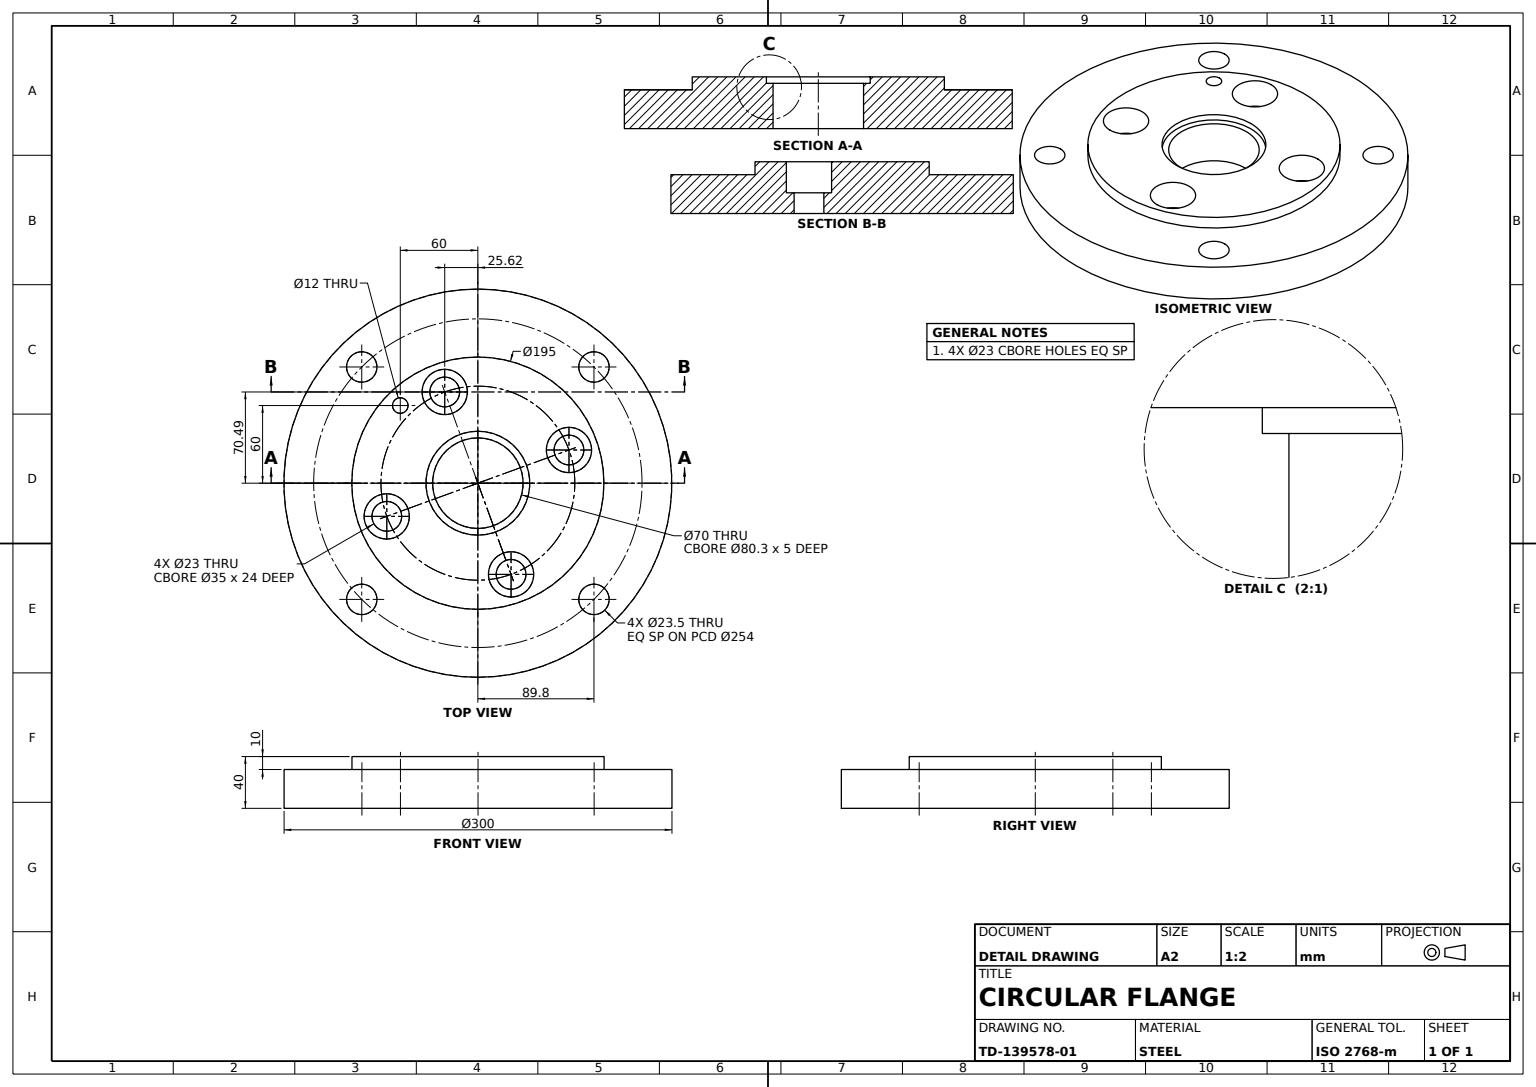
from build123d import *

# Parameters (mm, degrees)
FLANGE_DISC_SKETCH_300_R         = 150
FLANGE_DISC_300X40_DEPTH         = 40
BORE_SKETCH_70_R                 = 35
BORE_70_THROUGH_DEPTH            = 40
BORE_RECESS_SKETCH_80_3_R        = 40.15
BORE_RECESS_SKETCH_80_3_R_2      = 35
BORE_RECESS_80_3X5_DEPTH         = 5
RAISED_FACE_STEP_SKETCH_R        = 150
RAISED_FACE_STEP_SKETCH_R_2      = 97.5
RAISED_FACE_STEP_195X10_DEPTH    = 10
OUTER_BOLT_HOLES_SKETCH_PCD254_R = 11.75
OUTER_BOLT_HOLES_PCD254_DEPTH    = 215.242852856
INNER_HOLES_SKETCH_R             = 17.5
INNER_HOLES_CUT_24_DEEP_DEPTH    = 24
INNER_HOLE_SECONDARY_SKETCH_R    = 11.5
INNER_HOLE_SECONDARY_CUT_DEPTH   = 216.870331449
SMALL_HOLE_SKETCH_12_R           = 6
SMALL_HOLE_12_DEPTH              = 216.870331449


with BuildPart() as part:
    # Flange Disc Sketch Ø300 → Flange Disc Ø300x40 (new body)
    with BuildSketch(Plane(origin=(0, 0, 0), x_dir=(1, 0, 0), z_dir=(0, 1, 0))):
        with Locations(Location((0, 0, 0), (0, 0, 270))):
            Circle(FLANGE_DISC_SKETCH_300_R)
    extrude(amount=-FLANGE_DISC_300X40_DEPTH)

    # Bore Sketch Ø70 → Bore Ø70 Through (cut)
    with BuildSketch(Plane(origin=(0, 0, 0), x_dir=(1, 0, 0), z_dir=(0, 1, 0))):
        with Locations(Location((0, 0, 0), (0, 0, 270))):
            Circle(BORE_SKETCH_70_R)
    extrude(amount=-BORE_70_THROUGH_DEPTH, mode=Mode.SUBTRACT)

    # Bore Recess Sketch Ø80.3 → Bore Recess Ø80.3x5 (cut)
    with BuildSketch(Plane(origin=(0, 0, 0), x_dir=(1, 0, 0), z_dir=(0, 1, 0))):
        with Locations(Location((0, 0, 0), (0, 0, 270))):
            Circle(BORE_RECESS_SKETCH_80_3_R)
        with Locations(Location((0, 0, 0), (0, 0, 270))):
            Circle(BORE_RECESS_SKETCH_80_3_R_2, mode=Mode.SUBTRACT)
    extrude(amount=-BORE_RECESS_80_3X5_DEPTH, mode=Mode.SUBTRACT)

    # Raised Face Step Sketch → Raised Face Step Ø195x10 (cut)
    with BuildSketch(Plane(origin=(0, 0, 0), x_dir=(1, 0, 0), z_dir=(0, 1, 0))):
        with Locations(Location((0, 0, 0), (0, 0, 270))):
            Circle(RAISED_FACE_STEP_SKETCH_R)
        with Locations(Location((0, 0, 0), (0, 0, 270))):
            Circle(RAISED_FACE_STEP_SKETCH_R_2, mode=Mode.SUBTRACT)
    extrude(amount=-RAISED_FACE_STEP_195X10_DEPTH, mode=Mode.SUBTRACT)

    # Outer Bolt Holes Sketch PCD254 → Outer Bolt Holes PCD254 (cut, through all)
    with BuildSketch(Plane(origin=(0, -10, 0), x_dir=(1, 0, 0), z_dir=(0, 1, 0))):
        with Locations(Location((89.802561211, 89.802561211, 0), (0, 0, 270))):
            Circle(OUTER_BOLT_HOLES_SKETCH_PCD254_R)
        with Locations(Location((-89.802561211, 89.802561211, 0), (0, 0, 90))):
            Circle(OUTER_BOLT_HOLES_SKETCH_PCD254_R)
        with Locations(Location((-89.802561211, -89.802561211, 0), (0, 0, 270))):
            Circle(OUTER_BOLT_HOLES_SKETCH_PCD254_R)
        with Locations(Location((89.802561211, -89.802561211, 0), (0, 0, 90))):
            Circle(OUTER_BOLT_HOLES_SKETCH_PCD254_R)
    extrude(amount=-OUTER_BOLT_HOLES_PCD254_DEPTH, mode=Mode.SUBTRACT)

    # Inner Holes Sketch → Inner Holes Cut 24 Deep (cut)
    with BuildSketch(Plane(origin=(0, 0, 0), x_dir=(1, 0, 0), z_dir=(0, 1, 0))):
        with Locations(Location((-70.476946559, -25.651510749, 0), (0, 0, 270))):
            Circle(INNER_HOLES_SKETCH_R)
        with Locations(Location((70.476946559, 25.651510749, 0), (0, 0, 270))):
            Circle(INNER_HOLES_SKETCH_R)
        with Locations(Location((-25.616759959, 70.489585112, 0), (0, 0, 270))):
            Circle(INNER_HOLES_SKETCH_R)
        with Locations(Location((25.686255305, -70.464290874, 0), (0, 0, 270))):
            Circle(INNER_HOLES_SKETCH_R)
    extrude(amount=-INNER_HOLES_CUT_24_DEEP_DEPTH, mode=Mode.SUBTRACT)

    # Inner Hole Secondary Sketch → Inner Hole Secondary Cut (cut, through all)
    with BuildSketch(Plane(origin=(0, 0, 0), x_dir=(1, 0, 0), z_dir=(0, 1, 0))):
        with Locations(Location((70.476946559, 25.651510749, 0), (0, 0, 270))):
            Circle(INNER_HOLE_SECONDARY_SKETCH_R)
        with Locations(Location((-70.407451213, -25.626216512, 0), (0, 0, 270))):
            Circle(INNER_HOLE_SECONDARY_SKETCH_R)
        with Locations(Location((-25.616759959, 70.489585112, 0), (0, 0, 270))):
            Circle(INNER_HOLE_SECONDARY_SKETCH_R)
        with Locations(Location((25.686255305, -70.464290874, 0), (0, 0, 270))):
            Circle(INNER_HOLE_SECONDARY_SKETCH_R)
    extrude(amount=-INNER_HOLE_SECONDARY_CUT_DEPTH, mode=Mode.SUBTRACT)

    # Small Hole Sketch Ø12 → Small Hole Ø12 (cut, through all)
    with BuildSketch(Plane(origin=(0, 0, 0), x_dir=(1, 0, 0), z_dir=(0, 1, 0))):
        with Locations(Location((-60, 60, 0), (0, 0, 270))):
            Circle(SMALL_HOLE_SKETCH_12_R)
    extrude(amount=-SMALL_HOLE_12_DEPTH, mode=Mode.SUBTRACT)


solid = part.part
